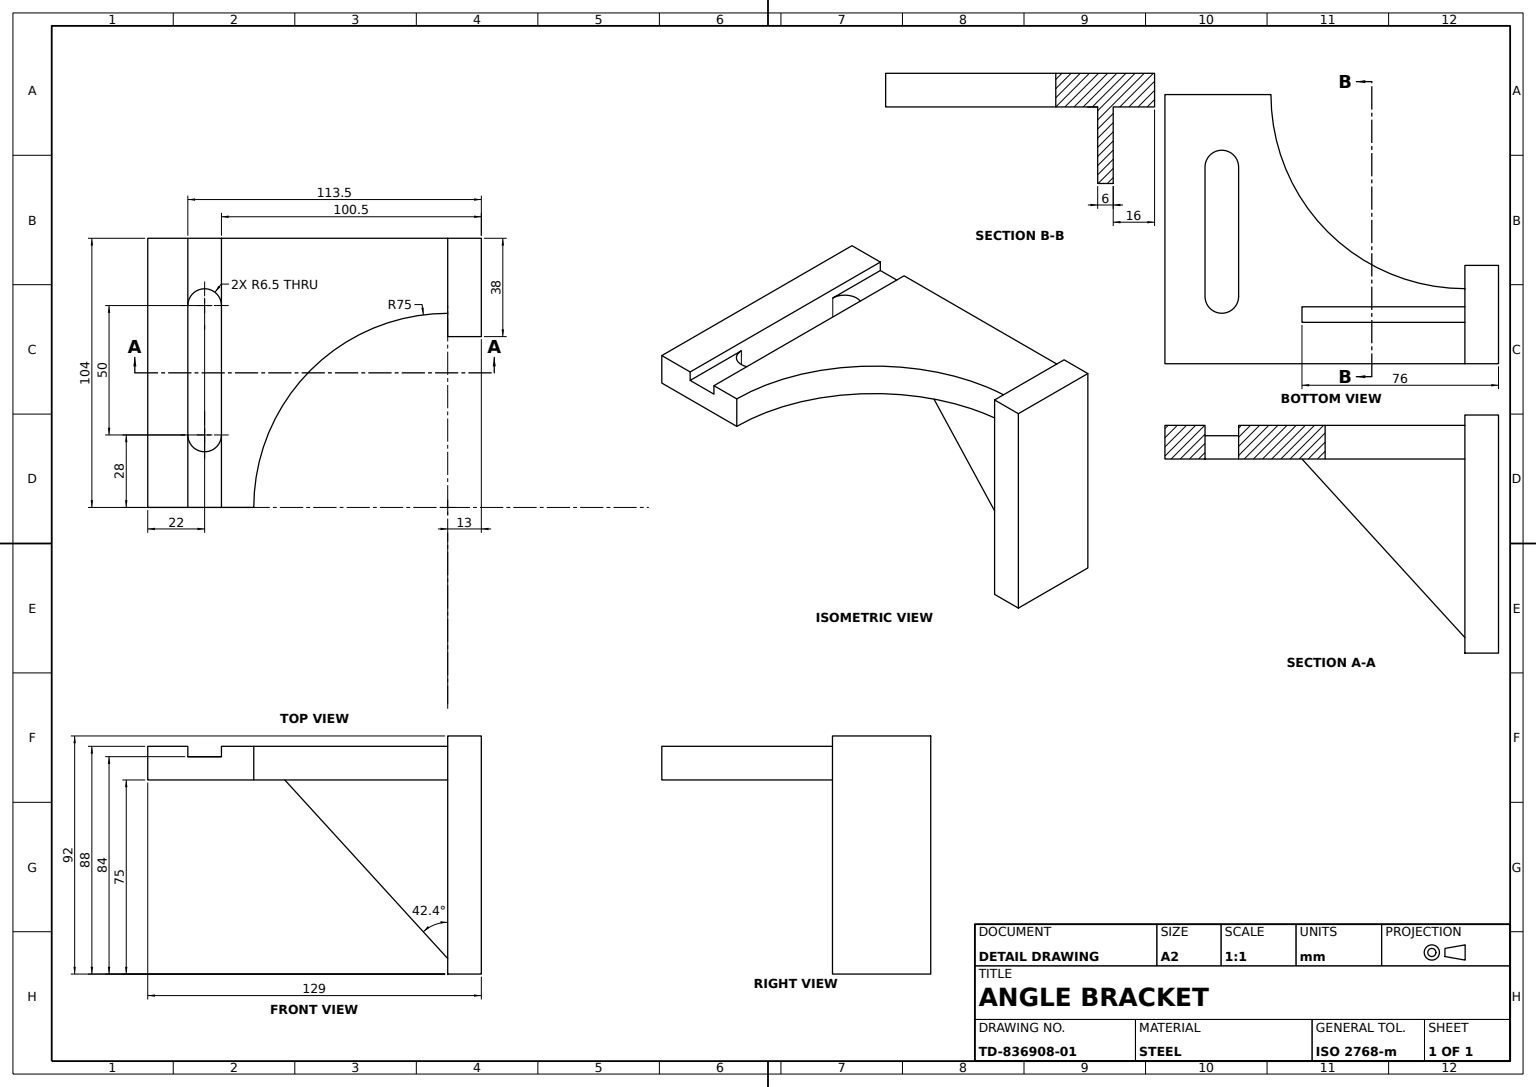
from build123d import *

# Parameters (mm, degrees)
BASE_PLATE_SKETCH_W     = 38
BASE_PLATE_SKETCH_H     = 92
BASE_PLATE_DEPTH        = 13
MAIN_BODY_104MM_DEPTH   = 104
CURVED_RELIEF_CUT_DEPTH = 13
SLOT_CUT_DEPTH          = 13
GUSSET_BOSS_38MM_DEPTH  = 38
NOTCH_CUT_A_DEPTH       = 16
NOTCH_CUT_B_DEPTH       = 16


with BuildPart() as part:
    # Base Plate Sketch → Base Plate (new body)
    with BuildSketch(Plane.XY):
        with Locations((19, -46)):
            Rectangle(BASE_PLATE_SKETCH_W, BASE_PLATE_SKETCH_H)
    extrude(amount=BASE_PLATE_DEPTH)

    # Main Body Profile Sketch → Main Body 104mm (add)
    with BuildSketch(Plane.ZY):
        Polygon((13, -4), (100.5, -4), (100.5, -8), (113.5, -8), (113.5, -4), (129, -4), (129, -17), (13, -17), align=None)
    extrude(amount=-MAIN_BODY_104MM_DEPTH)

    # Curved Relief Sketch → Curved Relief Cut (cut)
    with BuildSketch(Plane.XZ.offset(17)):
        with BuildLine():
            Line((104, 88), (104, 13))
            Line((104, 13), (29, 13))
            ThreePointArc((29, 13), (50.966991411, 66.033008589), (104, 88))
        make_face()
    extrude(amount=-CURVED_RELIEF_CUT_DEPTH, mode=Mode.SUBTRACT)

    # Slot Sketch → Slot Cut (cut)
    with BuildSketch(Plane.XZ.offset(17)):
        with BuildLine():
            Line((26, 113.5), (76, 113.5))
            ThreePointArc((76, 113.5), (82.5, 107), (76, 100.5))
            Line((76, 100.5), (26, 100.5))
            ThreePointArc((26, 100.5), (19.5, 107), (26, 113.5))
        make_face()
    extrude(amount=-SLOT_CUT_DEPTH, mode=Mode.SUBTRACT)

    # Gusset Boss Sketch → Gusset Boss 38mm (add)
    with BuildSketch(Plane.ZY):
        Polygon((13, -17), (76, -17), (13, -86), align=None)
    extrude(amount=-GUSSET_BOSS_38MM_DEPTH)

    # Notch Cut A Sketch → Notch Cut A (cut)
    with BuildSketch(Plane(origin=(38, 0, 0), x_dir=(0, 0, -1), z_dir=(1, 0, 0))):
        Polygon((-76, -17), (-13, -17), (-13, -86), align=None)
    extrude(amount=-NOTCH_CUT_A_DEPTH, mode=Mode.SUBTRACT)

    # Notch Cut B Sketch → Notch Cut B (cut)
    with BuildSketch(Plane.ZY):
        Polygon((76, -17), (13, -86), (13, -17), align=None)
    extrude(amount=-NOTCH_CUT_B_DEPTH, mode=Mode.SUBTRACT)


solid = part.part
